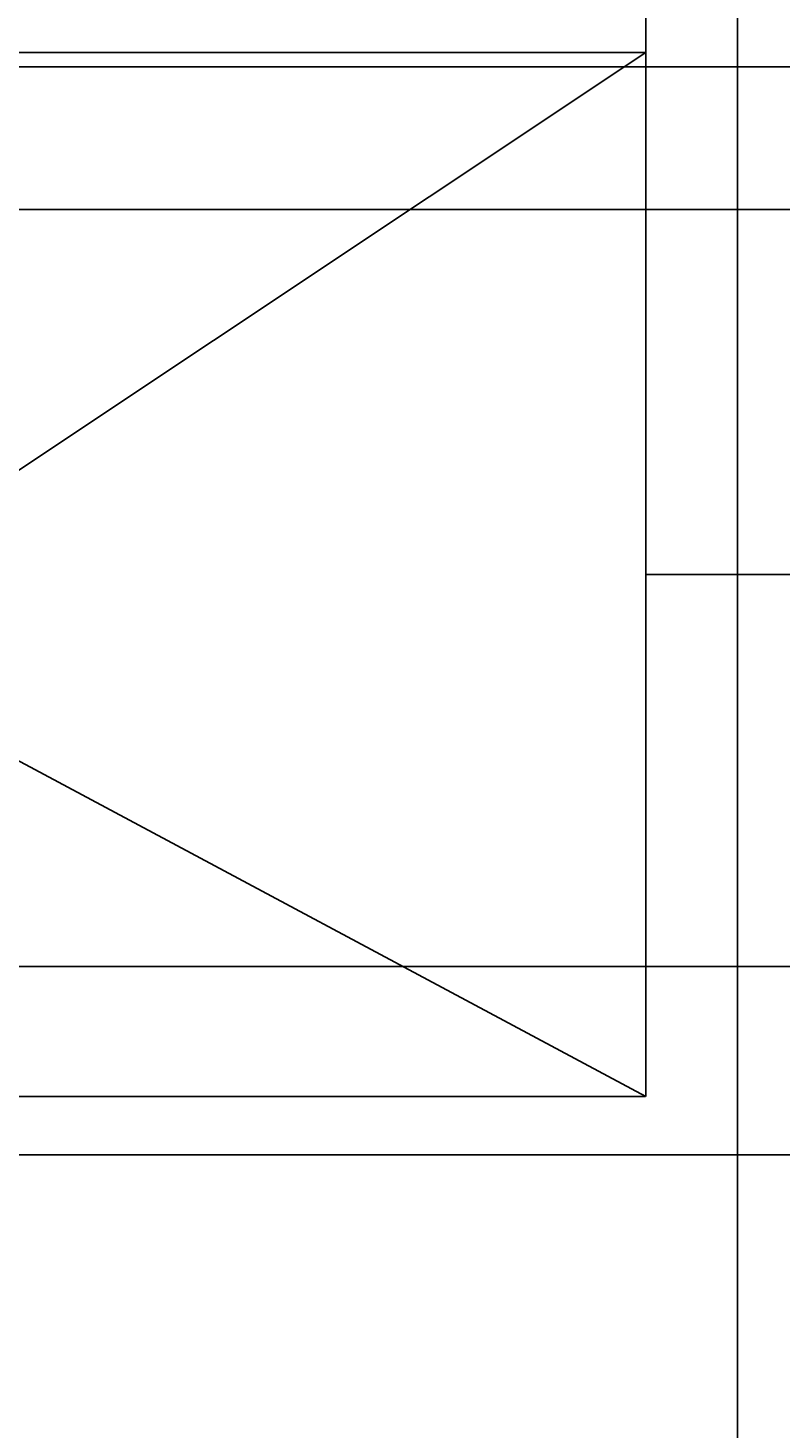
# Model space of a CAD drawing. Units: inches. Extents: x 35362 to 73946, y 43607 to 67532.
# Tile 122 of 134: x 51049 to 51337, y 48793 to 49329. Entities that reach past the tile are written whole.
import ezdxf

# ---------------------------------------------------------------- set-up
doc = ezdxf.new("R2010")
doc.units = ezdxf.units.IN
doc.header["$MEASUREMENT"] = 0
doc.layers.add('A-ANNO-DIMS', color=2, linetype='Continuous', lineweight=18)
doc.layers.add('E-SYMB', color=1, linetype='Continuous', lineweight=25)
doc.styles.get("Standard").update_dxf_attribs({"font": 'arial.ttf'})
doc.dimstyles.get("Standard").update_dxf_attribs({"dimtxt": 0.18, "dimasz": 0.18, "dimexe": 0.18, "dimexo": 0.0625, "dimgap": 0.09, "dimtad": 0, "dimtih": 1, "dimtoh": 1, "dimdec": 4, "dimzin": 0, "dimdsep": 46, "dimtxsty": 'Standard', "dimcen": 0.09, "dimadec": 0, "dimazin": 0, "dimtfac": 1, "dimtdec": 4, "dimtofl": 0, "dimtmove": 0, "dimatfit": 3, "dimfxl": 1, "dimtolj": 1, "dimtzin": 0, "dimarcsym": 0})

# ---------------------------------------------------------------- blocks, each defined once
blk = doc.blocks.new('*D11')
at = {"layer": 'A-ANNO-DIMS', "color": 0, "lineweight": -2, "transparency": 16777216}
for p, q in [((47978.66, 56028.77), (47978.66, 43606.68)), ((53109.76, 56028.77), (53109.76, 43606.68)), ((47978.84, 43606.86), (50543.87, 43606.86)), ((53109.58, 43606.86), (50544.55, 43606.86))]:
    blk.add_line(p, q, dxfattribs=at)
at = {"layer": 'A-ANNO-DIMS', "color": 0, "transparency": 16777216}
for points in [[(47978.84, 43606.89), (47978.84, 43606.83), (47978.66, 43606.86)], [(53109.58, 43606.89), (53109.58, 43606.83), (53109.76, 43606.86)]]:
    blk.add_solid(points, dxfattribs=at)
at = {"layer": 'Defpoints', "color": 0, "transparency": 16777216}
for p in [(47978.66, 56028.84), (53109.76, 56028.84), (53109.76, 43606.86)]:
    blk.add_point(p, dxfattribs=at)
at = {"layer": 'A-ANNO-DIMS', "color": 0, "transparency": 16777216, "insert": (50544.21, 43606.86), "char_height": 0.18, "attachment_point": 5}
blk.add_mtext('\\A1;5131', dxfattribs=at)
blk = doc.blocks.new('*D17')
at = {"layer": 'A-ANNO-DIMS', "color": 0, "lineweight": -2, "transparency": 16777216}
for p, q in [((49923.31, 61293.22), (49923.31, 43606.68)), ((51913.93, 61293.22), (51913.93, 43606.68)), ((49923.49, 43606.86), (50918.16, 43606.86)), ((51913.75, 43606.86), (50919.07, 43606.86))]:
    blk.add_line(p, q, dxfattribs=at)
at = {"layer": 'A-ANNO-DIMS', "color": 0, "transparency": 16777216}
for points in [[(49923.49, 43606.89), (49923.49, 43606.83), (49923.31, 43606.86)], [(51913.75, 43606.89), (51913.75, 43606.83), (51913.93, 43606.86)]]:
    blk.add_solid(points, dxfattribs=at)
at = {"layer": 'Defpoints', "color": 0, "transparency": 16777216}
for p in [(49923.31, 61293.29), (51913.93, 61293.29), (51913.93, 43606.86)]:
    blk.add_point(p, dxfattribs=at)
at = {"layer": 'A-ANNO-DIMS', "color": 0, "transparency": 16777216, "insert": (50918.62, 43606.86), "char_height": 0.18, "attachment_point": 5}
blk.add_mtext('\\A1;1990.6', dxfattribs=at)
blk = doc.blocks.new('*D40')
at = {"layer": 'A-ANNO-DIMS', "color": 0, "lineweight": -2, "transparency": 16777216}
for p, q in [((56873.54, 53351.53), (35361.77, 53351.53)), ((35361.95, 53351.35), (35361.95, 51333.28)), ((35361.95, 49314.85), (35361.95, 51332.92)), ((51806.45, 49314.67), (35361.77, 49314.67))]:
    blk.add_line(p, q, dxfattribs=at)
at = {"layer": 'A-ANNO-DIMS', "color": 0, "transparency": 16777216}
for points in [[(35361.92, 53351.35), (35361.98, 53351.35), (35361.95, 53351.53)], [(35361.92, 49314.85), (35361.98, 49314.85), (35361.95, 49314.67)]]:
    blk.add_solid(points, dxfattribs=at)
at = {"layer": 'Defpoints', "color": 0, "transparency": 16777216}
for p in [(35361.95, 53351.53), (56873.6, 53351.53), (51806.52, 49314.67)]:
    blk.add_point(p, dxfattribs=at)
at = {"layer": 'A-ANNO-DIMS', "color": 0, "transparency": 16777216, "insert": (35361.95, 51333.1), "char_height": 0.18, "attachment_point": 5}
blk.add_mtext('\\A1;4036.9', dxfattribs=at)
blk = doc.blocks.new('*D67')
at = {"layer": 'A-ANNO-DIMS', "color": 0, "lineweight": -2, "transparency": 16777216}
for p, q in [((56873.54, 53351.53), (35361.77, 53351.53)), ((35361.95, 53351.35), (35361.95, 49400.89)), ((35361.95, 45450.07), (35361.95, 49400.53)), ((53793.58, 45449.89), (35361.77, 45449.89))]:
    blk.add_line(p, q, dxfattribs=at)
at = {"layer": 'A-ANNO-DIMS', "color": 0, "transparency": 16777216}
for points in [[(35361.92, 53351.35), (35361.98, 53351.35), (35361.95, 53351.53)], [(35361.92, 45450.07), (35361.98, 45450.07), (35361.95, 45449.89)]]:
    blk.add_solid(points, dxfattribs=at)
at = {"layer": 'Defpoints', "color": 0, "transparency": 16777216}
for p in [(35361.95, 53351.53), (56873.6, 53351.53), (53793.64, 45449.89)]:
    blk.add_point(p, dxfattribs=at)
at = {"layer": 'A-ANNO-DIMS', "color": 0, "transparency": 16777216, "insert": (35361.95, 49400.71), "char_height": 0.18, "attachment_point": 5}
blk.add_mtext('\\A1;7901.6', dxfattribs=at)
blk = doc.blocks.new('*D84')
at = {"layer": 'A-ANNO-DIMS', "color": 0, "lineweight": -2, "transparency": 16777216}
for p, q in [((55540.23, 49259.94), (35361.77, 49259.94)), ((35361.95, 49259.76), (35361.95, 49115.14)), ((35361.95, 48970.16), (35361.95, 49114.78)), ((55540.23, 48969.98), (35361.77, 48969.98))]:
    blk.add_line(p, q, dxfattribs=at)
at = {"layer": 'A-ANNO-DIMS', "color": 0, "transparency": 16777216}
for points in [[(35361.92, 49259.76), (35361.98, 49259.76), (35361.95, 49259.94)], [(35361.92, 48970.16), (35361.98, 48970.16), (35361.95, 48969.98)]]:
    blk.add_solid(points, dxfattribs=at)
at = {"layer": 'Defpoints', "color": 0, "transparency": 16777216}
for p in [(35361.95, 49259.94), (55540.3, 49259.94), (55540.3, 48969.98)]:
    blk.add_point(p, dxfattribs=at)
at = {"layer": 'A-ANNO-DIMS', "color": 0, "transparency": 16777216, "insert": (35361.95, 49114.96), "char_height": 0.18, "attachment_point": 5}
blk.add_mtext('\\A1;289.96', dxfattribs=at)
blk = doc.blocks.new('*D85')
at = {"layer": 'A-ANNO-DIMS', "color": 0, "lineweight": -2, "transparency": 16777216}
for p, q in [((50952.66, 49098.43), (50952.66, 67531.69)), ((50952.84, 67531.51), (51118.73, 67531.51)), ((51285.41, 67531.51), (51119.52, 67531.51)), ((51285.59, 49320.14), (51285.59, 67531.69))]:
    blk.add_line(p, q, dxfattribs=at)
at = {"layer": 'A-ANNO-DIMS', "color": 0, "transparency": 16777216}
for points in [[(50952.84, 67531.54), (50952.84, 67531.48), (50952.66, 67531.51)], [(51285.41, 67531.54), (51285.41, 67531.48), (51285.59, 67531.51)]]:
    blk.add_solid(points, dxfattribs=at)
at = {"layer": 'Defpoints', "color": 0, "transparency": 16777216}
for p in [(51285.59, 67531.51), (51285.59, 49320.08), (50952.66, 49098.37)]:
    blk.add_point(p, dxfattribs=at)
at = {"layer": 'A-ANNO-DIMS', "color": 0, "transparency": 16777216, "insert": (51119.13, 67531.51), "char_height": 0.18, "attachment_point": 5}
blk.add_mtext('\\A1;332.9', dxfattribs=at)
blk = doc.blocks.new('*D86')
at = {"layer": 'A-ANNO-DIMS', "color": 0, "lineweight": -2, "transparency": 16777216}
for p, q in [((51285.53, 49320.08), (35361.77, 49320.08)), ((35361.95, 49319.9), (35361.95, 49120.26)), ((35361.95, 48920.26), (35361.95, 49119.9)), ((51285.53, 48920.08), (35361.77, 48920.08))]:
    blk.add_line(p, q, dxfattribs=at)
at = {"layer": 'A-ANNO-DIMS', "color": 0, "transparency": 16777216}
for points in [[(35361.92, 49319.9), (35361.98, 49319.9), (35361.95, 49320.08)], [(35361.92, 48920.26), (35361.98, 48920.26), (35361.95, 48920.08)]]:
    blk.add_solid(points, dxfattribs=at)
at = {"layer": 'Defpoints', "color": 0, "transparency": 16777216}
for p in [(35361.95, 49320.08), (51285.59, 49320.08), (51285.59, 48920.08)]:
    blk.add_point(p, dxfattribs=at)
at = {"layer": 'A-ANNO-DIMS', "color": 0, "transparency": 16777216, "insert": (35361.95, 49120.08), "char_height": 0.18, "attachment_point": 5}
blk.add_mtext('\\A1;400.0', dxfattribs=at)
blk = doc.blocks.new('*D89')
at = {"layer": 'A-ANNO-DIMS', "color": 0, "lineweight": -2, "transparency": 16777216}
for p, q in [((53707.72, 48897.74), (35361.77, 48897.74)), ((35361.95, 48897.56), (35361.95, 48303.16)), ((35361.95, 47708.4), (35361.95, 48302.8)), ((53707.72, 47708.22), (35361.77, 47708.22))]:
    blk.add_line(p, q, dxfattribs=at)
at = {"layer": 'A-ANNO-DIMS', "color": 0, "transparency": 16777216}
for points in [[(35361.92, 48897.56), (35361.98, 48897.56), (35361.95, 48897.74)], [(35361.92, 47708.4), (35361.98, 47708.4), (35361.95, 47708.22)]]:
    blk.add_solid(points, dxfattribs=at)
at = {"layer": 'Defpoints', "color": 0, "transparency": 16777216}
for p in [(53707.78, 48897.74), (35361.95, 47708.22), (53707.78, 47708.22)]:
    blk.add_point(p, dxfattribs=at)
at = {"layer": 'A-ANNO-DIMS', "color": 0, "transparency": 16777216, "insert": (35361.95, 48302.98), "char_height": 0.18, "attachment_point": 5}
blk.add_mtext('\\A1;1189.5', dxfattribs=at)
blk = doc.blocks.new('*D107')
at = {"layer": 'A-ANNO-DIMS', "color": 0, "lineweight": -2, "transparency": 16777216}
for p, q in [((50139.56, 59850.01), (50139.56, 43606.68)), ((51320.81, 59850.01), (51320.81, 43606.68)), ((50139.74, 43606.86), (50729.73, 43606.86)), ((51320.63, 43606.86), (50730.64, 43606.86))]:
    blk.add_line(p, q, dxfattribs=at)
at = {"layer": 'A-ANNO-DIMS', "color": 0, "transparency": 16777216}
for points in [[(50139.74, 43606.89), (50139.74, 43606.83), (50139.56, 43606.86)], [(51320.63, 43606.89), (51320.63, 43606.83), (51320.81, 43606.86)]]:
    blk.add_solid(points, dxfattribs=at)
at = {"layer": 'Defpoints', "color": 0, "transparency": 16777216}
for p in [(50139.56, 59850.08), (51320.81, 59850.08), (51320.81, 43606.86)]:
    blk.add_point(p, dxfattribs=at)
at = {"layer": 'A-ANNO-DIMS', "color": 0, "transparency": 16777216, "insert": (50730.19, 43606.86), "char_height": 0.18, "attachment_point": 5}
blk.add_mtext('\\A1;1181.3', dxfattribs=at)

msp = doc.modelspace()

# ---------------------------------------------------------------- linework, layer by layer
at = {"layer": 'E-SYMB'}
for p, q in [((51285.595, 49320.079), (50952.662, 49098.368)), ((51285.595, 49120.079), (51285.595, 49320.079)), ((51714.196, 49120.079), (51285.595, 49120.079)), ((51285.595, 49120.079), (51285.595, 48920.079)), ((50952.662, 49098.368), (51285.595, 48920.079))]:
    msp.add_line(p, q, dxfattribs=at)

# ---------------------------------------------------------------- dimensions: what is measured, and where the dimension line sits
at = {"layer": 'A-ANNO-DIMS'}
for base, p1, p2, override, picture, middle in [((51285.595, 67531.512), (50952.662, 49098.368), (51285.595, 49320.079), {"dimdec": 1, "dimlfac": 1, "dimrnd": 0, "dimzin": 0, "dimdsep": 46, "dimlunit": 2}, '*D85', (51119.128, 67531.512)), ((51913.931, 43606.859), (49923.307, 61293.286), (51913.931, 61293.286), {"dimdec": 1, "dimlfac": 1, "dimrnd": 0, "dimzin": 0, "dimdsep": 46, "dimlunit": 2}, '*D17', (50918.619, 43606.859)), ((51320.8133, 43606.859), (50139.5627, 59850.0769), (51320.8133, 59850.0769), {"dimdec": 1, "dimlfac": 1, "dimrnd": 0, "dimzin": 0, "dimdsep": 46, "dimlunit": 2}, '*D107', (50730.188, 43606.859)), ((53109.76, 43606.859), (47978.665, 56028.836), (53109.76, 56028.836), {"dimdec": 0, "dimlfac": 1, "dimrnd": 0, "dimzin": 0, "dimdsep": 46, "dimlunit": 2}, '*D11', (50544.212, 43606.859))]:
    dim = msp.add_linear_dim(base=base, p1=p1, p2=p2, dimstyle='Standard', override=override, dxfattribs=at)
    dim.commit()
    dim.dimension.update_dxf_attribs({"geometry": picture, "text_midpoint": middle})
for base, p1, p2, override, picture, middle in [((35361.949, 53351.529), (51806.517, 49314.669), (56873.602, 53351.529), {"dimdec": 1, "dimlfac": 1, "dimrnd": 0, "dimzin": 0, "dimdsep": 46, "dimlunit": 2}, '*D40', (35361.949, 51333.099)), ((35361.949, 53351.529), (53793.638, 45449.894), (56873.602, 53351.529), {"dimdec": 1, "dimlfac": 1, "dimrnd": 0, "dimzin": 0, "dimdsep": 46, "dimlunit": 2}, '*D67', (35361.949, 49400.712)), ((35361.949, 49320.079), (51285.595, 48920.079), (51285.595, 49320.079), {"dimdec": 1, "dimlfac": 1, "dimrnd": 0, "dimzin": 0, "dimdsep": 46, "dimlunit": 2}, '*D86', (35361.949, 49120.079)), ((35361.9491, 49259.9353), (55540.2972, 48969.9796), (55540.2972, 49259.9353), {"dimdec": 2, "dimlfac": 1, "dimrnd": 0, "dimzin": 0, "dimdsep": 46, "dimlunit": 2}, '*D84', (35361.9491, 49114.9575)), ((35361.949, 47708.216), (53707.781, 48897.738), (53707.781, 47708.216), {"dimdec": 1, "dimlfac": 1, "dimrnd": 0, "dimzin": 0, "dimdsep": 46, "dimlunit": 2}, '*D89', (35361.949, 48302.977))]:
    dim = msp.add_linear_dim(base=base, p1=p1, p2=p2, angle=90, dimstyle='Standard', override=override, dxfattribs=at)
    dim.commit()
    dim.dimension.update_dxf_attribs({"geometry": picture, "text_midpoint": middle})

doc.saveas('drawing.dxf')
